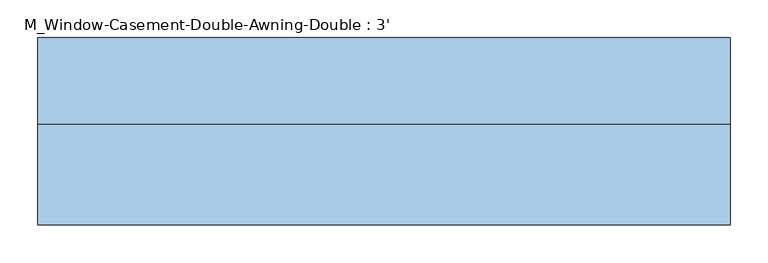
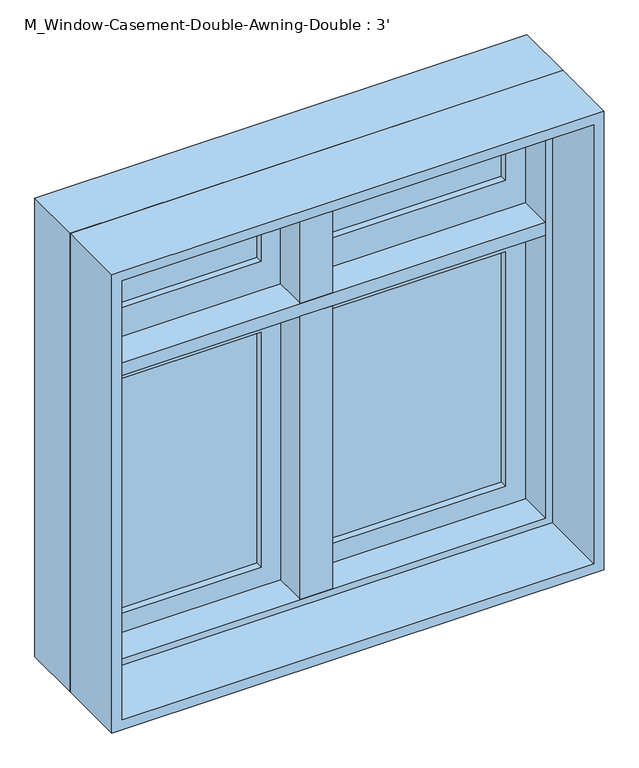
"""IFC4 building model written with IfcOpenShell, lengths in millimetres: window geometry, M_Window-Casement-Double-Awning-Double : 3'."""

from ifc_helpers import new_model, si_unit, frame, origin, place, context, project, spatial, polyline, outline, extrude, faceted_brep, source, transform, mapped, element, save


def m_window_casement_double_awning_double_3_6fa9dbfe(model_context):
    return source(origin(), model_context, "Body", "SolidModel", [
        faceted_brep([(425.45, 82.55, 1768.25), (425.45, 19.05, 1768.25), (-425.45, 19.05, 1768.25), (-425.45, 82.55, 1768.25), (444.5, 133.35, 1787.3), (444.5, 82.55, 1787.3), (-444.5, 82.55, 1787.3), (-444.5, 133.35, 1787.3), (457.2, 19.05, 1800.0), (457.2, 133.35, 1800.0), (-457.2, 133.35, 1800.0), (-457.2, 19.05, 1800.0), (-425.45, 19.05, 931.75), (-425.45, 82.55, 931.75), (-444.5, 82.55, 912.7), (-444.5, 133.35, 912.7), (-457.2, 133.35, 900.0), (-457.2, 19.05, 900.0), (425.45, 19.05, 931.75), (425.45, 82.55, 931.75), (444.5, 82.55, 912.7), (444.5, 133.35, 912.7), (457.2, 133.35, 900.0), (457.2, 19.05, 900.0)], [[[0, 1, 2, 3]], [[4, 5, 6, 7]], [[8, 9, 10, 11]], [[3, 2, 12, 13]], [[7, 6, 14, 15]], [[11, 10, 16, 17]], [[13, 12, 18, 19]], [[15, 14, 20, 21]], [[17, 16, 22, 23]], [[11, 17, 23, 8], [1, 18, 12, 2]], [[19, 18, 1, 0]], [[5, 20, 14, 6], [3, 13, 19, 0]], [[21, 20, 5, 4]], [[23, 22, 9, 8]], [[9, 22, 16, 10], [7, 15, 21, 4]]]),
        extrude(outline(polyline([(1800.0, -457.2), (900.0, -457.2), (900.0, 457.2), (1800.0, 457.2), (1800.0, -457.2)]), holes=[polyline([(1780.95, 438.15), (919.05, 438.15), (919.05, -438.15), (1780.95, -438.15), (1780.95, 438.15)])]), frame((0.0, -114.3, 0.0), z_axis=(0.0, 1.0, 0.0), x_axis=(0.0, 0.0, 1.0)), (0.0, 0.0, 1.0), 133.35),
        extrude(outline(polyline([(912.7, 444.5), (1487.3, 444.5), (1487.3, 9.525), (912.7, 9.525), (912.7, 444.5)]), holes=[polyline([(969.85, 66.675), (1430.15, 66.675), (1430.15, 387.35), (969.85, 387.35), (969.85, 66.675)])]), frame((0.0, 82.55, 0.0), z_axis=(0.0, 1.0, 0.0), x_axis=(0.0, 0.0, 1.0)), (0.0, 0.0, 1.0), 44.45),
        extrude(outline(polyline([(1487.3, -444.5), (912.7, -444.5), (912.7, -9.525), (1487.3, -9.525), (1487.3, -444.5)]), holes=[polyline([(1430.15, -66.675), (969.85, -66.675), (969.85, -387.35), (1430.15, -387.35), (1430.15, -66.675)])]), frame((0.0, 82.55, 0.0), z_axis=(0.0, 1.0, 0.0), x_axis=(0.0, 0.0, 1.0)), (0.0, 0.0, 1.0), 44.45),
        extrude(outline(polyline([(387.35, 114.3), (387.35, 107.95), (66.675, 107.95), (66.675, 114.3), (387.35, 114.3)])), frame((0.0, 0.0, 969.85), z_axis=(0.0, 0.0, 1.0), x_axis=(1.0, 0.0, 0.0)), (0.0, 0.0, 1.0), 460.3),
        extrude(outline(polyline([(66.675, 95.25), (66.675, 101.6), (387.35, 101.6), (387.35, 95.25), (66.675, 95.25)])), frame((0.0, 0.0, 969.85), z_axis=(0.0, 0.0, 1.0), x_axis=(1.0, 0.0, 0.0)), (0.0, 0.0, 1.0), 460.3),
        extrude(outline(polyline([(-66.675, 114.3), (-66.675, 107.95), (-387.35, 107.95), (-387.35, 114.3), (-66.675, 114.3)])), frame((0.0, 0.0, 969.85), z_axis=(0.0, 0.0, 1.0), x_axis=(1.0, 0.0, 0.0)), (0.0, 0.0, 1.0), 460.3),
        extrude(outline(polyline([(-387.35, 95.25), (-387.35, 101.6), (-66.675, 101.6), (-66.675, 95.25), (-387.35, 95.25)])), frame((0.0, 0.0, 969.85), z_axis=(0.0, 0.0, 1.0), x_axis=(1.0, 0.0, 0.0)), (0.0, 0.0, 1.0), 460.3),
        faceted_brep([(9.525, 133.35, 1487.3), (-9.525, 133.35, 1487.3), (-9.525, 82.55, 1487.3), (-30.1625, 82.55, 1487.3), (-30.1625, 19.05, 1487.3), (30.1625, 19.05, 1487.3), (30.1625, 82.55, 1487.3), (9.525, 82.55, 1487.3), (9.525, 133.35, 912.7), (9.525, 82.55, 912.7), (-9.525, 82.55, 912.7), (-9.525, 133.35, 912.7), (-9.525, 82.55, 931.75), (-30.1625, 82.55, 931.75), (-30.1625, 19.05, 931.75), (30.1625, 19.05, 931.75), (30.1625, 82.55, 931.75), (9.525, 82.55, 931.75)], [[[0, 1, 2, 3, 4, 5, 6, 7]], [[8, 9, 10, 11]], [[1, 0, 8, 11]], [[2, 1, 11, 10, 12]], [[3, 2, 12, 13]], [[4, 3, 13, 14]], [[5, 4, 14, 15]], [[6, 5, 15, 16]], [[7, 6, 16, 17]], [[0, 7, 17, 9, 8]], [[17, 12, 10, 9]], [[12, 17, 16, 15, 14, 13]]]),
        extrude(outline(polyline([(-66.675, 114.3), (-66.675, 107.95), (-387.35, 107.95), (-387.35, 114.3), (-66.675, 114.3)])), frame((0.0, 0.0, 1569.85), z_axis=(0.0, 0.0, 1.0), x_axis=(1.0, 0.0, 0.0)), (0.0, 0.0, 1.0), 160.3),
        extrude(outline(polyline([(-387.35, 95.25), (-387.35, 101.6), (-66.675, 101.6), (-66.675, 95.25), (-387.35, 95.25)])), frame((0.0, 0.0, 1569.85), z_axis=(0.0, 0.0, 1.0), x_axis=(1.0, 0.0, 0.0)), (0.0, 0.0, 1.0), 160.3),
        extrude(outline(polyline([(444.5, 133.35), (444.5, 82.55), (425.45, 82.55), (425.45, 19.05), (-425.45, 19.05), (-425.45, 82.55), (-444.5, 82.55), (-444.5, 133.35), (444.5, 133.35)])), frame((0.0, 0.0, 1487.3), z_axis=(0.0, 0.0, 1.0), x_axis=(1.0, 0.0, 0.0)), (0.0, 0.0, 1.0), 25.4),
        faceted_brep([(9.525, 82.55, 1787.3), (9.525, 133.35, 1787.3), (-9.525, 133.35, 1787.3), (-9.525, 82.55, 1787.3), (-9.525, 82.55, 1512.7), (-9.525, 133.35, 1512.7), (9.525, 133.35, 1512.7), (9.525, 82.55, 1512.7), (30.1625, 82.55, 1512.7), (30.1625, 19.05, 1512.7), (-30.1625, 19.05, 1512.7), (-30.1625, 82.55, 1512.7), (-30.1625, 82.55, 1768.25), (-9.525, 82.55, 1768.25), (-30.1625, 19.05, 1768.25), (30.1625, 19.05, 1768.25), (30.1625, 82.55, 1768.25), (9.525, 82.55, 1768.25)], [[[0, 1, 2, 3]], [[4, 5, 6, 7, 8, 9, 10, 11]], [[4, 11, 12, 13]], [[11, 10, 14, 12]], [[10, 9, 15, 14]], [[9, 8, 16, 15]], [[8, 7, 17, 16]], [[1, 0, 17, 7, 6]], [[2, 1, 6, 5]], [[3, 2, 5, 4, 13]], [[17, 13, 12, 14, 15, 16]], [[13, 17, 0, 3]]]),
        extrude(outline(polyline([(1787.3, 9.525), (1512.7, 9.525), (1512.7, 444.5), (1787.3, 444.5), (1787.3, 9.525)]), holes=[polyline([(1730.15, 387.35), (1569.85, 387.35), (1569.85, 66.675), (1730.15, 66.675), (1730.15, 387.35)])]), frame((0.0, 82.55, 0.0), z_axis=(0.0, 1.0, 0.0), x_axis=(0.0, 0.0, 1.0)), (0.0, 0.0, 1.0), 44.45),
        extrude(outline(polyline([(1512.7, -9.525), (1787.3, -9.525), (1787.3, -444.5), (1512.7, -444.5), (1512.7, -9.525)]), holes=[polyline([(1569.85, -387.35), (1730.15, -387.35), (1730.15, -66.675), (1569.85, -66.675), (1569.85, -387.35)])]), frame((0.0, 82.55, 0.0), z_axis=(0.0, 1.0, 0.0), x_axis=(0.0, 0.0, 1.0)), (0.0, 0.0, 1.0), 44.45),
        extrude(outline(polyline([(66.675, 114.3), (387.35, 114.3), (387.35, 107.95), (66.675, 107.95), (66.675, 114.3)])), frame((0.0, 0.0, 1569.85), z_axis=(0.0, 0.0, 1.0), x_axis=(1.0, 0.0, 0.0)), (0.0, 0.0, 1.0), 160.3),
        extrude(outline(polyline([(387.35, 95.25), (66.675, 95.25), (66.675, 101.6), (387.35, 101.6), (387.35, 95.25)])), frame((0.0, 0.0, 1569.85), z_axis=(0.0, 0.0, 1.0), x_axis=(1.0, 0.0, 0.0)), (0.0, 0.0, 1.0), 160.3),
    ])


if __name__ == "__main__":
    model = new_model("IFC4")
    model_context = context("Model", 3, world=origin())
    ifc_project = project(units=[si_unit("LENGTHUNIT", "METRE", prefix="MILLI")], contexts=[model_context])
    site = spatial("IfcSite", under=ifc_project)
    building = spatial("IfcBuilding", under=site)
    placement = place(None, origin())
    m_window_casement_double_awning_double_3_shape = m_window_casement_double_awning_double_3_6fa9dbfe(model_context)
    element("IfcWindow", 1, ObjectType="M_Window-Casement-Double-Awning-Double : 3'", at=placement, inside=building, context=model_context, shape_type="MappedRepresentation", body=[
        mapped(m_window_casement_double_awning_double_3_shape, transform((0.0, 0.0, 0.0), x_axis=(1.0, 0.0, 0.0), y_axis=(0.0, 1.0, 0.0), z_axis=(0.0, 0.0, 1.0))),
    ])
    save(model, "model.ifc")

# Revit data of these elements
# Type "M_Window-Casement-Double-Awning-Double : 3'"
#   Type Mark = "31"
#   Fire Rating = "0.5h"
#   Assembly Code = "B2020100"
#   Analytic Construction = "Double glazing - domestic"
#   Window Inset [instance default] = 0' - 0"
#   Wall Thickness [instance default] = 0' - 5.90551"
#   Interior Wall Closure [instance default] = 0' - 2.15551"
#   Half Width = 1' - 6"
#   Visual Light Transmittance = 0.81
#   Transom Height = 0' - 11.81102"
#   Thermal Resistance (R) = 0.319569 (m²·K)/W
#   Solar Heat Gain Coefficient = 0.76
#   Rough Width = 3' - 0.59055"
#   Rough Height = 3' - 0.02362"
#   Open Window Height = 1' - 11.62205"
#   Frame Extension [instance default] = 0' - 0 1/4"
#   Height = 2' - 11.43307"
#   Heat Transfer Coefficient (U) = 3.12929 W/(m²·K)
#   Exterior Wall Closure [instance default] = 0' - 1.25197"
#   Extension Jamb [instance default] = 0' - 2.15551"
#   Default Sill Height = 2' - 11.43307"
#   Width = 3' - 0"
#   Top Muntin Visibility = yes
#   Bottom Muntin Visibility = yes
#   Interior Trim Visibility [instance default] = yes
#   Exterior Trim Visibility [instance default] = yes
#   Extension Jamb Visibility [instance default] = yes
#   Interior Trim Material = Wood - Stained
#   Muntin Pattern = M_Muntin Pattern_2x2 : M_Muntin Pattern_2x2
#   Interior Trim = M_Trim-Window-Interior-Flat : Picture Frame
#   Interior Frame Material = Wood - Stained
#   Glass Panel Material = Glass
#   Exterior Trim Material = Clad - White
#   Exterior Trim = M_Trim-Window-Exterior-Flat : with Sill
#   Exterior Frame Material = Clad - White
#   Wall Closure = (empty or 0)
# Element 1 (IfcWindow, "M_Window-Casement-Double-Awning-Double : 3'")
#   Wall Thickness = 0' - 9"
#   Extension Jamb = 0' - 5 1/4"
#   Materials on its faces: "Wood - Stained", "Glass", "Clad - White"
# Materials
#   "Wood - Stained": class "Wood", colour RGB 224 178 126, transparency 0, Cost = 0
#   "Glass": class "Glass", colour RGB 0 128 192, transparency 0.9, Description = "Soda Lime Glass", Cost = 0
#   "Clad - White": class "Wood", colour RGB 242 242 238, transparency 0, Cost = 0
